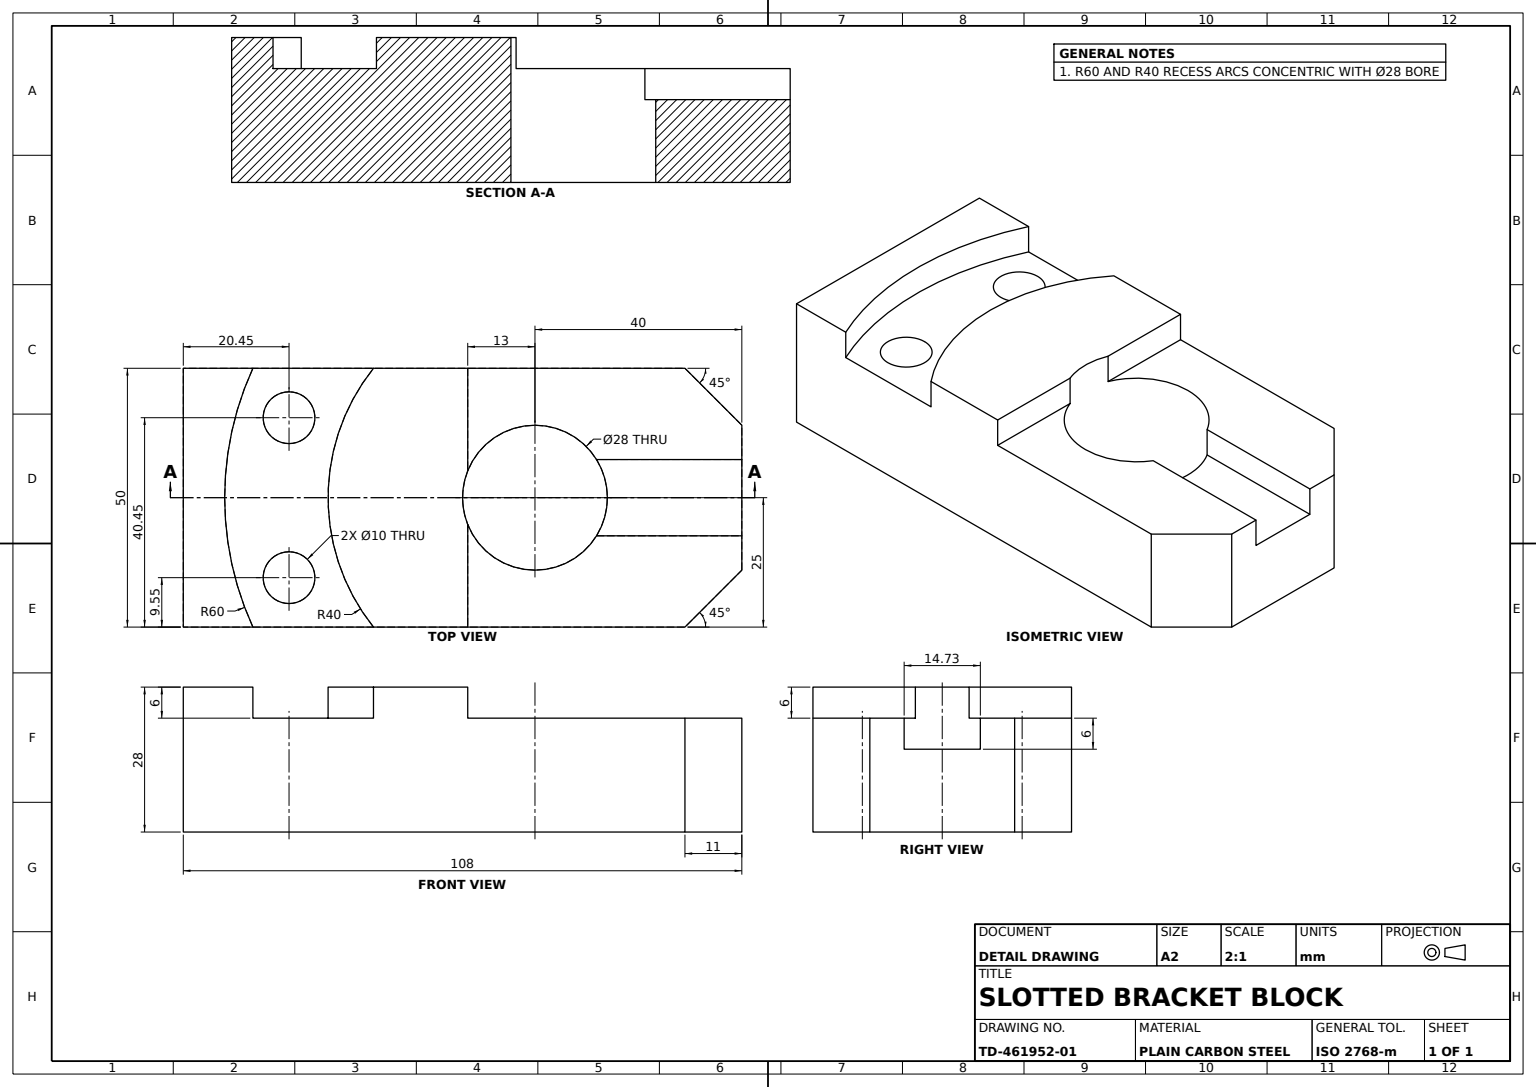
from build123d import *

# Parameters (mm, degrees)
BASE_BLOCK_SKETCH_W        = 108
BASE_BLOCK_SKETCH_H        = 50
BASE_BLOCK_108X50X28_DEPTH = 14
END_CHAMFER_11X45DEG_SIZE  = 11
THROUGH_BORE_SKETCH_R      = 14
THROUGH_BORE_DEPTH         = 28
SLOT_RECESS_6_DEEP_DEPTH   = 6
ARC_RECESS_6_DEEP_DEPTH    = 6
ARC_HOLES_SKETCH_R         = 5
HOLES_2XD10_ON_R100_DEPTH  = 22
GROOVE_6_DEEP_DEPTH        = 6


with BuildPart() as part:
    # Base Block Sketch → Base Block 108x50x28 (new, symmetric)
    with BuildSketch(Plane(origin=(0, 0, 0), x_dir=(1, 0, 0), z_dir=(0, 1, 0))):
        Rectangle(BASE_BLOCK_SKETCH_W, BASE_BLOCK_SKETCH_H)
    extrude(amount=BASE_BLOCK_108X50X28_DEPTH, both=True)

    # End Chamfer 11x45deg
    end_chamfer_11x45deg_edges = [part.edges().sort_by_distance(p)[0] for p in [
        (54, 0, 25),
        (54, 0, -25),
    ]]
    chamfer(end_chamfer_11x45deg_edges, length=END_CHAMFER_11X45DEG_SIZE)

    # Through Bore Sketch → Through Bore (cut)
    with BuildSketch(Plane(origin=(0, 14, 0), x_dir=(1, 0, 0), z_dir=(0, 1, 0))):
        with Locations(Location((14, 0, 0), (0, 0, 270))):
            Circle(THROUGH_BORE_SKETCH_R)
    extrude(amount=-THROUGH_BORE_DEPTH, mode=Mode.SUBTRACT)

    # Slot Recess Sketch → Slot Recess 6 Deep (cut)
    with BuildSketch(Plane(origin=(0, 14, 0), x_dir=(1, 0, 0), z_dir=(0, 1, 0))):
        Polygon((1, 25), (1, -25), (43, -25), (54, -14), (54, 14), (43, 25), align=None)
    extrude(amount=-SLOT_RECESS_6_DEEP_DEPTH, mode=Mode.SUBTRACT)

    # Arc Recess Sketch → Arc Recess 6 Deep (cut)
    with BuildSketch(Plane(origin=(0, 14, 0), x_dir=(1, 0, 0), z_dir=(0, 1, 0))):
        with BuildLine():
            Line((-40.543560573, -25), (-17.224989992, -25))
            ThreePointArc((-17.224989992, -25), (-26, 0), (-17.224989992, 25))
            Line((-17.224989992, 25), (-40.543560573, 25))
            ThreePointArc((-40.543560573, 25), (-46, 0), (-40.543560573, -25))
        make_face()
    extrude(amount=-ARC_RECESS_6_DEEP_DEPTH, mode=Mode.SUBTRACT)

    # Arc Holes Sketch → Holes 2xD10 on R100 (cut)
    with BuildSketch(Plane(origin=(0, 8, 0), x_dir=(1, 0, 0), z_dir=(0, 1, 0))):
        with Locations(Location((-33.552825815, 15.450849719, 0), (0, 0, 270))):
            Circle(ARC_HOLES_SKETCH_R)
        with Locations(Location((-33.552825815, -15.450849719, 0), (0, 0, 270))):
            Circle(ARC_HOLES_SKETCH_R)
    extrude(amount=-HOLES_2XD10_ON_R100_DEPTH, mode=Mode.SUBTRACT)

    # Groove Sketch → Groove 6 Deep (cut)
    with BuildSketch(Plane(origin=(0, 8, 0), x_dir=(1, 0, 0), z_dir=(0, 1, 0))):
        with BuildLine():
            Line((25.904726429, 7.367325747), (54, 7.367325747))
            Line((54, 7.367325747), (54, -7.367325747))
            Line((54, -7.367325747), (25.904726429, -7.367325747))
            ThreePointArc((25.904726429, -7.367325747), (28, 0), (25.904726429, 7.367325747))
        make_face()
    extrude(amount=-GROOVE_6_DEEP_DEPTH, mode=Mode.SUBTRACT)


solid = part.part
